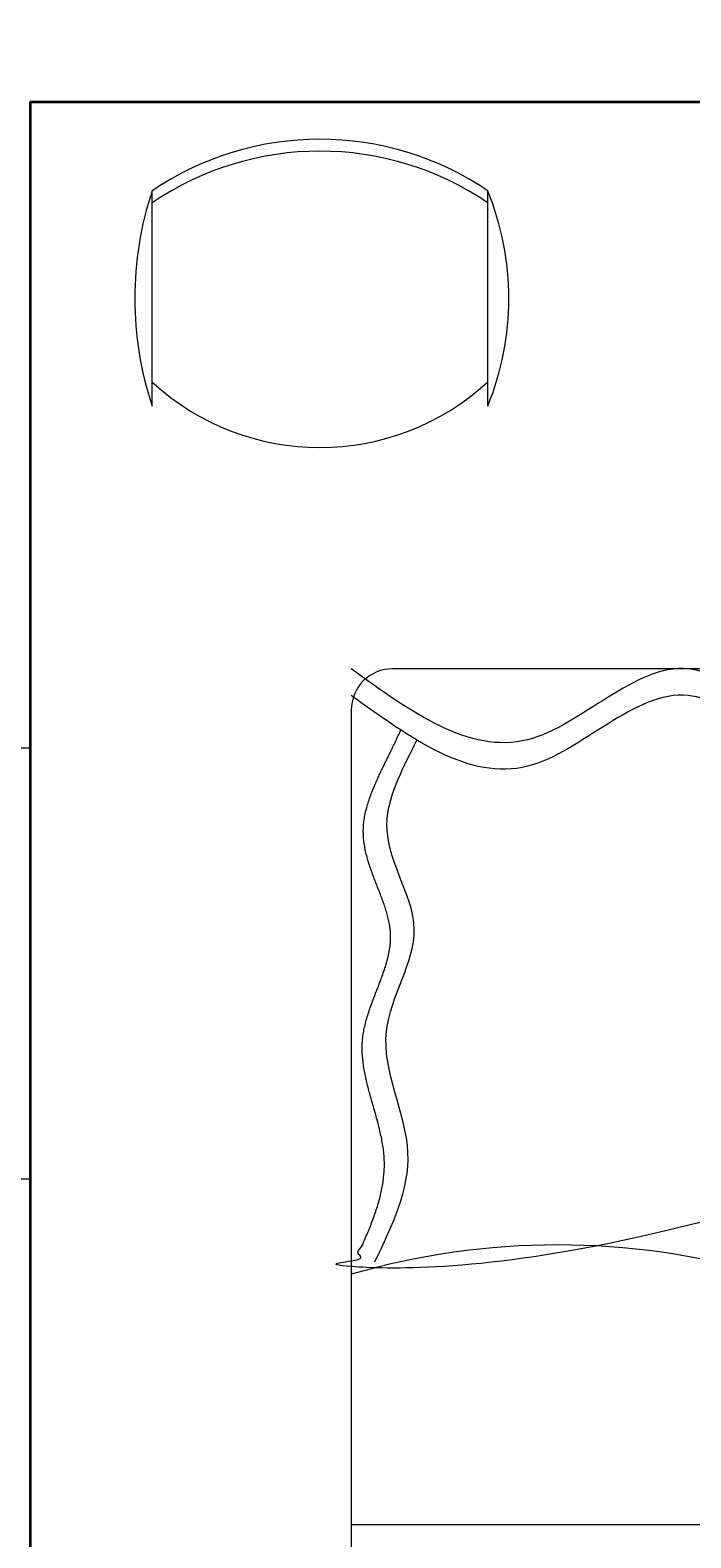
# Model space of a CAD drawing. Units: inches. Extents: x -61 to 1599, y -1316 to 257.
# Tile 52 of 204: x 88 to 143, y -408 to -282. Entities that reach past the tile are written whole.
import ezdxf

# ---------------------------------------------------------------- set-up
doc = ezdxf.new("R2010")
doc.units = ezdxf.units.IN
doc.header["$MEASUREMENT"] = 0
for name, color, linetype, lineweight in [('A-ANNO-DIMS', 2, 'Continuous', 18), ('FURNITURE', 83, 'Continuous', 18), ('WALLS', 4, 'Continuous', 35), ('WINDOWS', 220, 'Continuous', 18)]:
    doc.layers.add(name, color=color, linetype=linetype, lineweight=lineweight)
doc.styles.get("Standard").update_dxf_attribs({"font": 'arial.ttf'})
doc.dimstyles.get("Standard").update_dxf_attribs({"dimtxt": 0.18, "dimasz": 0.18, "dimexe": 0.18, "dimexo": 0.0625, "dimgap": 0.09, "dimtad": 0, "dimtih": 1, "dimtoh": 1, "dimdec": 0, "dimzin": 0, "dimdsep": 46, "dimlunit": 3, "dimtxsty": 'Standard', "dimcen": 0.09, "dimadec": 0, "dimazin": 0, "dimtfac": 1, "dimtdec": 0, "dimtofl": 0, "dimtmove": 0, "dimatfit": 3, "dimfxl": 1, "dimtolj": 1, "dimtzin": 0, "dimarcsym": 0})

# ---------------------------------------------------------------- blocks, each defined once
blk = doc.blocks.new('WIN-36IN')
for p, q in [((0, 4.5), (0, 9)), ((0, 9), (0, 0)), ((36, 9), (36, 0)), ((0, 5.26), (36, 5.26)), ((0, 4.5), (36, 4.5)), ((0, 4.5), (36, 4.5))]:
    blk.add_line(p, q)
blk = doc.blocks.new('BEDROOM-CHAIR')
for p, q in [((1.45, 3.47), (1.45, 21.47)), ((29.49, 3.47), (29.49, 21.47))]:
    blk.add_line(p, q)
for centre, radius, start, end in [((15.47, 0.83), 24.95, 55.8098, 124.1902), ((15.47, -0.17), 24.95, 55.8098, 124.1902), ((28.58, 12.47), 28.58, 161.6455, 198.3545), ((7.26, 12.47), 23.99, 337.9646, 22.0354), ((15.47, 20.69), 20.68, 227.332, 312.668)]:
    blk.add_arc(centre, radius, start, end)
blk = doc.blocks.new('BED-DOUBLE')
blk.add_line((1.27, 20.47), (70.26, 20.47))
blk.add_lwpolyline([(1.27, 88.54), (1.27, 3.45, 0.414214), (4.72, 0), (66.81, 0, 0.414214), (70.26, 3.45), (70.26, 88.54, 0.414214), (66.81, 91.99), (4.72, 91.99, 0.414214)], format="xyb", close=True)
blk.add_lwpolyline([(70.26, 41.39, -0.22309), (35.77, 41.39, 0.142156), (1.27, 41.39)], format="xyb")
for points, knots in [([(70.26, 91.99), (67.71, 89.38), (62.21, 83.76), (52.49, 96.72), (40.92, 82.74), (28.61, 96.74), (15.69, 81.53), (6.21, 88.41), (1.27, 91.99)], [0, 0, 0, 0, 9.176033, 19.753992, 33.150145, 45.209422, 59.881559, 75.764594, 75.764594, 75.764594, 75.764594]), ([(70.26, 89.76), (67.71, 87.16), (62.21, 81.54), (52.49, 94.5), (40.92, 80.52), (28.61, 94.52), (15.69, 79.31), (6.21, 86.19), (1.27, 89.76)], [0, 0, 0, 0, 9.176033, 19.753992, 33.150145, 45.209422, 59.881559, 75.764594, 75.764594, 75.764594, 75.764594]), ([(3.25, 42.44), (4.7, 45.45), (7.72, 51.72), (2.12, 61.25), (8.81, 70.52), (2.43, 77.93), (5.72, 83.91), (6.75, 86.04)], [0, 0, 0, 0, 8.27671, 17.241866, 24.903358, 33.244933, 38.427294, 38.427294, 38.427294, 38.427294])]:
    blk.add_open_spline(points, degree=3, knots=knots)
blk.add_open_spline([(5.01, 91.99), (4.99, 92.01), (4.96, 92.03), (4.94, 92.04)], degree=3)
blk.add_rational_spline([(70.26, 57.9), (59.86, 50.94), (48.6, 45.5), (36.68, 41.68), (36.46, 41.77), (36.25, 41.87), (36.03, 41.97), (24.6, 45.28), (12.69, 45.26), (1.27, 41.89), (2.72, 44.9), (5.74, 51.17), (0.14, 60.7), (6.83, 69.97), (0.11, 77.79), (4.35, 84.38), (5.4, 86.88)], [1, 0.993520320424, 0.993520320424, 1, 0.99997444972, 0.99997444972, 1, 0.973174868659, 0.973174868659, 1, 1, 1, 1, 1, 1, 1, 1], degree=3, knots=[0, 0, 0, 0, 0.279074, 0.279074, 0.279074, 0.296584, 0.296584, 0.296584, 0.865868, 0.865868, 0.865868, 9.142578, 18.107734, 25.769226, 34.110801, 40.441511, 40.441511, 40.441511, 40.441511])
blk = doc.blocks.new('*D687')
at = {"layer": 'A-ANNO-DIMS', "color": 0, "lineweight": -2, "transparency": 16777216}
for p, q in [((289.42, 181.68), (-61.08, 181.68)), ((-60.9, 181.5), (-60.9, -528.95)), ((-60.9, -1239.76), (-60.9, -529.32)), ((319.64, -1239.94), (-61.08, -1239.94))]:
    blk.add_line(p, q, dxfattribs=at)
at = {"layer": 'A-ANNO-DIMS', "color": 0, "transparency": 16777216}
for points in [[(-60.93, 181.5), (-60.87, 181.5), (-60.9, 181.68)], [(-60.93, -1239.76), (-60.87, -1239.76), (-60.9, -1239.94)]]:
    blk.add_solid(points, dxfattribs=at)
at = {"layer": 'DEFPOINTS', "color": 0, "transparency": 16777216}
for p in [(289.48, 181.68), (-60.9, -1239.94), (319.7, -1239.94)]:
    blk.add_point(p, dxfattribs=at)
at = {"layer": 'A-ANNO-DIMS', "color": 0, "transparency": 16777216, "insert": (-60.9, -529.13), "char_height": 0.18, "attachment_point": 5}
blk.add_mtext('\\A1;1421.6', dxfattribs=at)
blk = doc.blocks.new('*D699')
at = {"layer": 'A-ANNO-DIMS', "color": 0, "lineweight": -2, "transparency": 16777216}
for p, q in [((835.64, -167.17), (-61.08, -167.17)), ((-60.9, -167.35), (-60.9, -306.73)), ((-60.9, -446.47), (-60.9, -307.09)), ((841.64, -446.65), (-61.08, -446.65))]:
    blk.add_line(p, q, dxfattribs=at)
at = {"layer": 'A-ANNO-DIMS', "color": 0, "transparency": 16777216}
for points in [[(-60.93, -167.35), (-60.87, -167.35), (-60.9, -167.17)], [(-60.93, -446.47), (-60.87, -446.47), (-60.9, -446.65)]]:
    blk.add_solid(points, dxfattribs=at)
at = {"layer": 'DEFPOINTS', "color": 0, "transparency": 16777216}
for p in [(835.7, -167.17), (-60.9, -446.65), (841.7, -446.65)]:
    blk.add_point(p, dxfattribs=at)
at = {"layer": 'A-ANNO-DIMS', "color": 0, "transparency": 16777216, "insert": (-60.9, -306.91), "char_height": 0.18, "attachment_point": 5}
blk.add_mtext('\\A1;279.5', dxfattribs=at)
blk = doc.blocks.new('*D700')
at = {"layer": 'A-ANNO-DIMS', "color": 0, "lineweight": -2, "transparency": 16777216}
for p, q in [((14.7, -616.88), (14.7, 257.46)), ((14.88, 257.28), (96.77, 257.28)), ((179.57, 257.28), (97.68, 257.28)), ((179.75, -616.88), (179.75, 257.46))]:
    blk.add_line(p, q, dxfattribs=at)
at = {"layer": 'A-ANNO-DIMS', "color": 0, "transparency": 16777216}
for points in [[(14.88, 257.31), (14.88, 257.25), (14.7, 257.28)], [(179.57, 257.31), (179.57, 257.25), (179.75, 257.28)]]:
    blk.add_solid(points, dxfattribs=at)
at = {"layer": 'DEFPOINTS', "color": 0, "transparency": 16777216}
for p in [(179.75, 257.28), (14.7, -616.94), (179.75, -616.94)]:
    blk.add_point(p, dxfattribs=at)
at = {"layer": 'A-ANNO-DIMS', "color": 0, "transparency": 16777216, "insert": (97.23, 257.28), "char_height": 0.18, "attachment_point": 5}
blk.add_mtext('\\A1;165.05', dxfattribs=at)

msp = doc.modelspace()

# ---------------------------------------------------------------- linework, layer by layer
at = {"layer": 'WALLS'}
for q in [(87.7028, -432.3229), (235.0034, -288.3229)]:
    msp.add_line((87.7028, -288.3229), q, dxfattribs=at)

# ---------------------------------------------------------------- block references
at = {"layer": 'FURNITURE'}
for name, p in [('BEDROOM-CHAIR', (96.4434, -317.2179)), ('BED-DOUBLE', (113.2612, -427.6961))]:
    msp.add_blockref(name, p, dxfattribs=at)
at = {"layer": 'WINDOWS', "rotation": 90.00000000000006}
msp.add_blockref('WIN-36IN', (87.7029, -378.3189), dxfattribs=at)

# ---------------------------------------------------------------- dimensions: what is measured, and where the dimension line sits
at = {"layer": 'A-ANNO-DIMS'}
dim = msp.add_linear_dim(base=(179.7521, 257.2771), p1=(14.7028, -616.9446), p2=(179.7521, -616.9446), dimstyle='Standard', override={"dimdec": 2, "dimlfac": 1, "dimrnd": 0, "dimzin": 0, "dimdsep": 46, "dimlunit": 2}, dxfattribs=at)
dim.commit()
dim.dimension.update_dxf_attribs({"geometry": '*D700', "text_midpoint": (97.2274, 257.2771)})
for base, p1, p2, picture, middle in [((-60.8972, -1239.9446), (289.4807, 181.6771), (319.7028, -1239.9446), '*D687', (-60.8972, -529.1337)), ((-60.8972, -446.6462), (835.7028, -167.169), (841.7028, -446.6462), '*D699', (-60.8972, -306.9076))]:
    dim = msp.add_linear_dim(base=base, p1=p1, p2=p2, angle=90, dimstyle='Standard', override={"dimdec": 1, "dimlfac": 1, "dimrnd": 0, "dimzin": 0, "dimdsep": 46, "dimlunit": 2}, dxfattribs=at)
    dim.commit()
    dim.dimension.update_dxf_attribs({"geometry": picture, "text_midpoint": middle})

doc.saveas('drawing.dxf')
